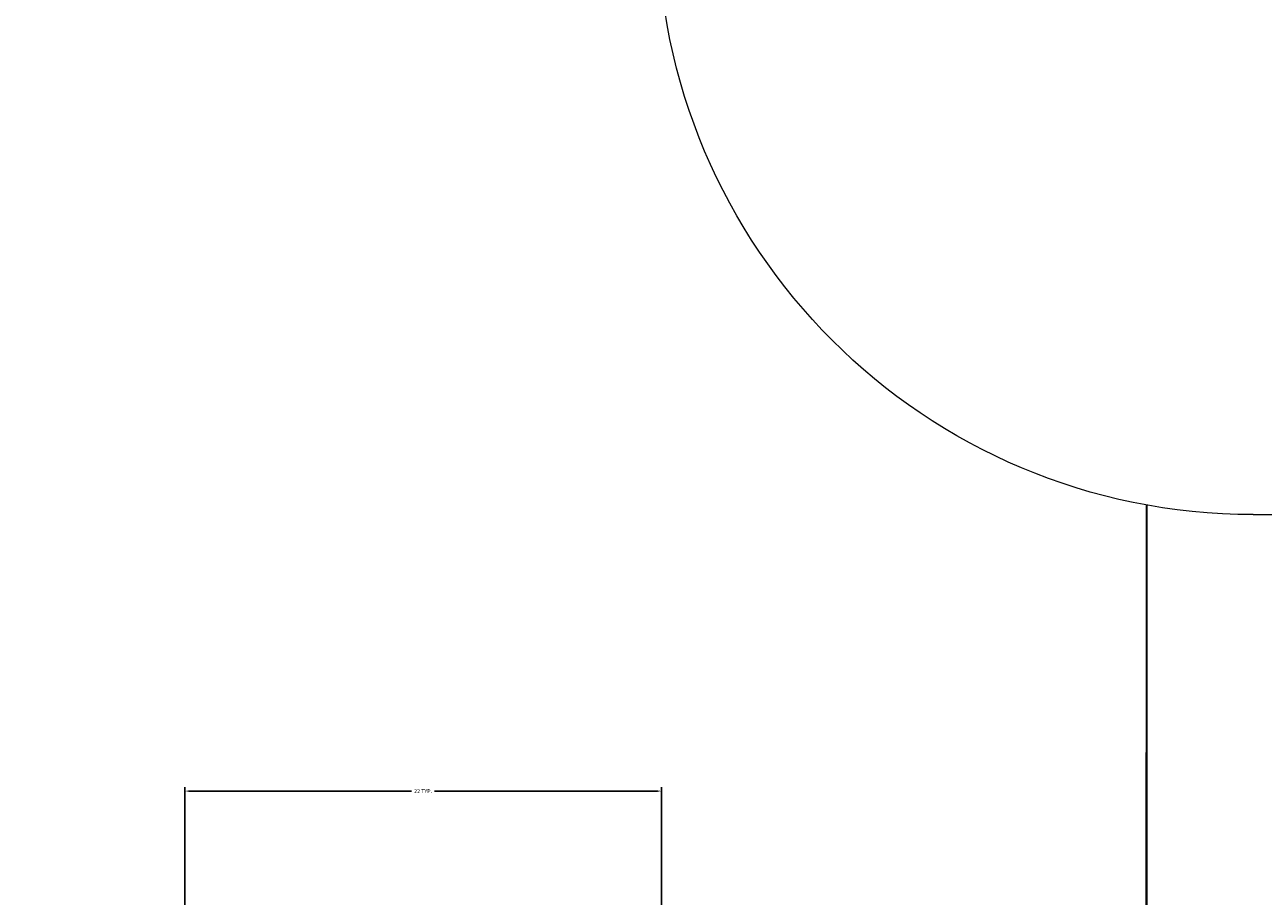
# Model space of a CAD drawing. Units: millimetres. Extents: x 27017497 to 27018854, y 7058029 to 7059154.
# Tile 58 of 91: x 27017980 to 27018038, y 7058369 to 7058409. Entities that reach past the tile are written whole.
import ezdxf

# ---------------------------------------------------------------- set-up
doc = ezdxf.new("R2010")
doc.units = ezdxf.units.MM
for name, color, linetype, lineweight in [('A-ANNO-DIMS', 2, 'Continuous', 18), ('A-DOOR', 4, 'Continuous', 20), ('A-WALL', 7, 'Continuous', 35)]:
    doc.layers.add(name, color=color, linetype=linetype, lineweight=lineweight)
doc.styles.get("Standard").update_dxf_attribs({"font": 'arial.ttf'})
doc.dimstyles.get("Standard").update_dxf_attribs({"dimtxt": 0.18, "dimasz": 0.18, "dimexe": 0.18, "dimexo": 0.0625, "dimgap": 0.09, "dimtad": 0, "dimtih": 1, "dimtoh": 1, "dimdec": 4, "dimzin": 0, "dimdsep": 46, "dimtxsty": 'Standard', "dimcen": 0.09, "dimadec": 0, "dimazin": 0, "dimtfac": 1, "dimtdec": 4, "dimtofl": 0, "dimtmove": 0, "dimatfit": 3, "dimfxl": 1, "dimtolj": 1, "dimtzin": 0, "dimarcsym": 0})

# ---------------------------------------------------------------- blocks, each defined once
blk = doc.blocks.new('*U2')
for p, q in [((0, 0), (0, -6)), ((40, 0), (40, -6))]:
    blk.add_line(p, q)
blk.add_lwpolyline([(0, 0), (0, 40), (1.75, 40), (1.75, 0)], close=True)
blk.add_arc((0, 0), 40, 0, 90)
blk = doc.blocks.new('*D28')
at = {"layer": 'A-ANNO-DIMS', "color": 0, "lineweight": -2, "transparency": 16777216}
for p, q in [((27017987.769, 7058367.649), (27017987.769, 7058373.769)), ((27018009.776, 7058367.649), (27018009.776, 7058373.769)), ((27017987.949, 7058373.589), (27017998.243, 7058373.589)), ((27018009.596, 7058373.589), (27017999.302, 7058373.589))]:
    blk.add_line(p, q, dxfattribs=at)
at = {"layer": 'A-ANNO-DIMS', "color": 0, "transparency": 16777216}
for points in [[(27017987.949, 7058373.619), (27017987.949, 7058373.559), (27017987.769, 7058373.589)], [(27018009.596, 7058373.619), (27018009.596, 7058373.559), (27018009.776, 7058373.589)]]:
    blk.add_solid(points, dxfattribs=at)
at = {"layer": 'Defpoints', "color": 0, "transparency": 16777216}
for p in [(27018009.776, 7058373.589), (27017987.769, 7058367.587), (27018009.776, 7058367.587)]:
    blk.add_point(p, dxfattribs=at)
at = {"layer": 'A-ANNO-DIMS', "color": 0, "transparency": 16777216, "insert": (27017998.772, 7058373.589), "char_height": 0.18, "attachment_point": 5}
blk.add_mtext('\\A1;22 TYP.', dxfattribs=at)
blk = doc.blocks.new('*D48')
at = {"layer": 'A-ANNO-DIMS', "color": 0, "lineweight": -2, "transparency": 16777216}
for p, q in [((27018463.498, 7058622.912), (27017497.536, 7058622.912)), ((27017497.716, 7058622.732), (27017497.716, 7058357.753)), ((27017497.716, 7058092.41), (27017497.716, 7058357.389)), ((27018555.129, 7058092.23), (27017497.536, 7058092.23))]:
    blk.add_line(p, q, dxfattribs=at)
at = {"layer": 'A-ANNO-DIMS', "color": 0, "transparency": 16777216}
for points in [[(27017497.686, 7058622.732), (27017497.746, 7058622.732), (27017497.716, 7058622.912)], [(27017497.686, 7058092.41), (27017497.746, 7058092.41), (27017497.716, 7058092.23)]]:
    blk.add_solid(points, dxfattribs=at)
at = {"layer": 'Defpoints', "color": 0, "transparency": 16777216}
for p in [(27018463.561, 7058622.912), (27017497.716, 7058092.23), (27018555.192, 7058092.23)]:
    blk.add_point(p, dxfattribs=at)
at = {"layer": 'A-ANNO-DIMS', "color": 0, "transparency": 16777216, "insert": (27017497.716, 7058357.571), "char_height": 0.18, "attachment_point": 5}
blk.add_mtext('\\A1;530.7', dxfattribs=at)

msp = doc.modelspace()

# ---------------------------------------------------------------- linework, layer by layer
at = {"layer": 'A-WALL'}
msp.add_line((27018032.166, 7058386.803), (27018032.166, 7058141.912), dxfattribs=at)
msp.add_lwpolyline([(27018032.178, 7058237.363), (27018032.178, 7058375.363)], dxfattribs=at)

# ---------------------------------------------------------------- block references
at = {"layer": 'A-DOOR', "xscale": -0.6870473523349573, "yscale": 0.6870473523349573, "zscale": 0.6870473523349573, "rotation": 90}
msp.add_blockref('*U2', (27018037.095, 7058413.839), dxfattribs=at)

# ---------------------------------------------------------------- dimensions: what is measured, and where the dimension line sits
at = {"layer": 'A-ANNO-DIMS'}
dim = msp.add_linear_dim(base=(27017497.716, 7058092.23), p1=(27018463.561, 7058622.912), p2=(27018555.192, 7058092.23), angle=90, dimstyle='Standard', override={"dimdec": 1, "dimlfac": 1, "dimrnd": 0, "dimzin": 0, "dimdsep": 46, "dimlunit": 2}, dxfattribs=at)
dim.commit()
dim.dimension.update_dxf_attribs({"geometry": '*D48', "text_midpoint": (27017497.716, 7058357.571)})
dim = msp.add_linear_dim(base=(27018009.776, 7058373.589), p1=(27017987.769, 7058367.587), p2=(27018009.776, 7058367.587), text='<> TYP.', dimstyle='Standard', override={"dimdec": 0, "dimlfac": 1, "dimrnd": 0, "dimzin": 0, "dimdsep": 46, "dimlunit": 2}, dxfattribs=at)
dim.commit()
dim.dimension.update_dxf_attribs({"geometry": '*D28', "text_midpoint": (27017998.772, 7058373.589)})

doc.saveas('drawing.dxf')
